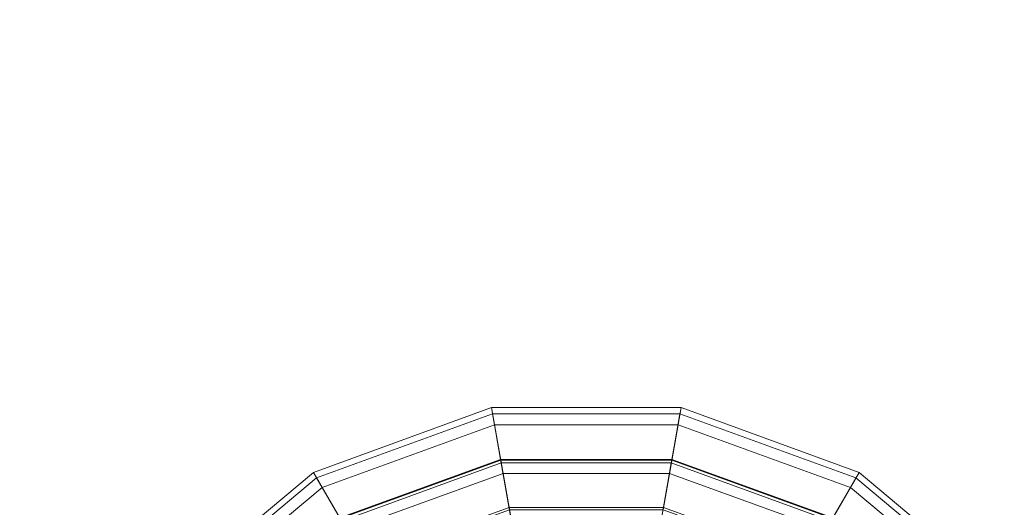
# Model space of a CAD drawing. Units: inches. Extents: x 375 to 1122, y 27 to 1069.
# Tile 122 of 155: x 717.857 to 720.301, y 892.201 to 893.412. Entities that reach past the tile are written whole.
import ezdxf

# ---------------------------------------------------------------- set-up
doc = ezdxf.new("R2010")
doc.units = ezdxf.units.IN
doc.layers.add('Furniture', color=30, linetype='Continuous', lineweight=18)

# ---------------------------------------------------------------- blocks, each defined once
blk = doc.blocks.new('A$C403C54AD')
for points in [[(1.160585, 0.881322, -0.028594), (1.158486, 0.883824, -0.031825), (1.150927, 0.874815, -0.031825), (1.153755, 0.873182, -0.028594)], [(1.158486, 0.883824, -0.031825), (1.180252, 0.857884, -0.028747), (1.180252, 0.857884, -0.028747), (1.150927, 0.874815, -0.031825)], [(1.160611, 0.881291, 0.131159), (1.158742, 0.883518, 0.117935), (1.151272, 0.874616, 0.117935), (1.15379, 0.873162, 0.131159)], [(1.158742, 0.883518, 0.117935), (1.159176, 0.883001, 0.089693), (1.151856, 0.874278, 0.089693), (1.151272, 0.874616, 0.117935)], [(1.159176, 0.883001, 0.089693), (1.162624, 0.878892, 0.071684), (1.156502, 0.871596, 0.071684), (1.151856, 0.874278, 0.089693)], [(1.153755, 0.873182, -0.028594), (1.150927, 0.874815, -0.031825), (1.146904, 0.863764, -0.031825), (1.15012, 0.863197, -0.028594)], [(1.150927, 0.874815, -0.031825), (1.180252, 0.857884, -0.028747), (1.180252, 0.857884, -0.028747), (1.146904, 0.863764, -0.031825)], [(1.15379, 0.873162, 0.131159), (1.151272, 0.874616, 0.117935), (1.147297, 0.863695, 0.117935), (1.15016, 0.86319, 0.131159)], [(1.151272, 0.874616, 0.117935), (1.151856, 0.874278, 0.089693), (1.147962, 0.863578, 0.089693), (1.147297, 0.863695, 0.117935)], [(1.151856, 0.874278, 0.089693), (1.156502, 0.871596, 0.071684), (1.153245, 0.862646, 0.071684), (1.147962, 0.863578, 0.089693)], [(1.167942, 0.864991, -0.02532), (1.153755, 0.873182, -0.028594), (1.15012, 0.863197, -0.028594), (1.166254, 0.860352, -0.02532)], [(1.158117, 0.870664, 0.140564), (1.15379, 0.873162, 0.131159), (1.15016, 0.86319, 0.131159), (1.155081, 0.862322, 0.140564)], [(1.153943, 0.873073, 0.117718), (1.156376, 0.871669, 0.130354), (1.153102, 0.862671, 0.130354), (1.150335, 0.863159, 0.117718)], [(1.154513, 0.872744, 0.090178), (1.153943, 0.873073, 0.117718), (1.150335, 0.863159, 0.117718), (1.150983, 0.863045, 0.090178)], [(1.158936, 0.87019, 0.073031), (1.154513, 0.872744, 0.090178), (1.150983, 0.863045, 0.090178), (1.156013, 0.862158, 0.073031)], [(1.15012, 0.863197, -0.028594), (1.146904, 0.863764, -0.031825), (1.146904, 0.852004, -0.031825), (1.15012, 0.852571, -0.028594)], [(1.146904, 0.863764, -0.031825), (1.180252, 0.857884, -0.028747), (1.180252, 0.857884, -0.028747), (1.146904, 0.852004, -0.031825)], [(1.15016, 0.86319, 0.131159), (1.147297, 0.863695, 0.117935), (1.147297, 0.852073, 0.117935), (1.15016, 0.852578, 0.131159)], [(1.147297, 0.863695, 0.117935), (1.147962, 0.863578, 0.089693), (1.147962, 0.85219, 0.089693), (1.147297, 0.852073, 0.117935)], [(1.147962, 0.863578, 0.089693), (1.153245, 0.862646, 0.071684), (1.153245, 0.853122, 0.071684), (1.147962, 0.85219, 0.089693)], [(1.166254, 0.860352, -0.02532), (1.15012, 0.863197, -0.028594), (1.15012, 0.852571, -0.028594), (1.166254, 0.855416, -0.02532)], [(1.155081, 0.862322, 0.140564), (1.15016, 0.86319, 0.131159), (1.15016, 0.852578, 0.131159), (1.155081, 0.853446, 0.140564)], [(1.150335, 0.863159, 0.117718), (1.153102, 0.862671, 0.130354), (1.153102, 0.853097, 0.130354), (1.150335, 0.852609, 0.117718)], [(1.150983, 0.863045, 0.090178), (1.150335, 0.863159, 0.117718), (1.150335, 0.852609, 0.117718), (1.150983, 0.852723, 0.090178)], [(1.156013, 0.862158, 0.073031), (1.150983, 0.863045, 0.090178), (1.150983, 0.852723, 0.090178), (1.156013, 0.85361, 0.073031)], [(1.146904, 0.852004, -0.031825), (1.180252, 0.857884, -0.028747), (1.180252, 0.857884, -0.028747), (1.150927, 0.840953, -0.031825)], [(1.150927, 0.840953, -0.031825), (1.180252, 0.857884, -0.028747), (1.180252, 0.857884, -0.028747), (1.158486, 0.831944, -0.031825)], [(1.166254, 0.855416, -0.02532), (1.15012, 0.852571, -0.028594), (1.153755, 0.842586, -0.028594), (1.167942, 0.850777, -0.02532)], [(1.156013, 0.85361, 0.073031), (1.150983, 0.852723, 0.090178), (1.154513, 0.843024, 0.090178), (1.158936, 0.845577, 0.073031)], [(1.147962, 0.85219, 0.089693), (1.153245, 0.853122, 0.071684), (1.156502, 0.844172, 0.071684), (1.151856, 0.84149, 0.089693)], [(1.155081, 0.853446, 0.140564), (1.15016, 0.852578, 0.131159), (1.15379, 0.842606, 0.131159), (1.158117, 0.845104, 0.140564)], [(1.150335, 0.852609, 0.117718), (1.153102, 0.853097, 0.130354), (1.156376, 0.844099, 0.130354), (1.153943, 0.842695, 0.117718)], [(1.15012, 0.852571, -0.028594), (1.146904, 0.852004, -0.031825), (1.150927, 0.840953, -0.031825), (1.153755, 0.842586, -0.028594)], [(1.15016, 0.852578, 0.131159), (1.147297, 0.852073, 0.117935), (1.151272, 0.841152, 0.117935), (1.15379, 0.842606, 0.131159)], [(1.150983, 0.852723, 0.090178), (1.150335, 0.852609, 0.117718), (1.153943, 0.842695, 0.117718), (1.154513, 0.843024, 0.090178)], [(1.147297, 0.852073, 0.117935), (1.147962, 0.85219, 0.089693), (1.151856, 0.84149, 0.089693), (1.151272, 0.841152, 0.117935)], [(1.151856, 0.84149, 0.089693), (1.156502, 0.844172, 0.071684), (1.162624, 0.836876, 0.071684), (1.159176, 0.832767, 0.089693)], [(1.153755, 0.842586, -0.028594), (1.150927, 0.840953, -0.031825), (1.158486, 0.831944, -0.031825), (1.160585, 0.834446, -0.028594)], [(1.15379, 0.842606, 0.131159), (1.151272, 0.841152, 0.117935), (1.158742, 0.83225, 0.117935), (1.160611, 0.834477, 0.131159)], [(1.151272, 0.841152, 0.117935), (1.151856, 0.84149, 0.089693), (1.159176, 0.832767, 0.089693), (1.158742, 0.83225, 0.117935)]]:
    blk.add_3dface(points)
at = {"linetype": 'ByBlock', "invisible_edges": 5}
for points in [[(1.149468, 0.81008, -0.008737), (1.140233, 0.794084, -0.008737), (1.080205, 0.810169, -0.008737), (1.080205, 0.828639, -0.008737)], [(1.132537, 0.780755, -0.02259), (1.149468, 0.81008, -0.013355), (1.080205, 0.828639, -0.013355), (1.080205, 0.794777, -0.02259)]]:
    blk.add_3dface(points, dxfattribs=at)
at = {"linetype": 'ByBlock'}
blk.add_3dface([(1.149468, 0.81008, -0.013355), (1.149468, 0.81008, -0.008737), (1.080205, 0.828639, -0.008737), (1.080205, 0.828639, -0.013355)], dxfattribs=at)

msp = doc.modelspace()

# ---------------------------------------------------------------- block references
at = {"layer": 'Furniture', "xscale": 39.9918517141215, "yscale": 39.9918517141215, "zscale": 39.9918517141215, "rotation": 270}
msp.add_blockref('A$C403C54AD', (684.9549, 938.3156, 0.024), dxfattribs=at)

doc.saveas('drawing.dxf')
